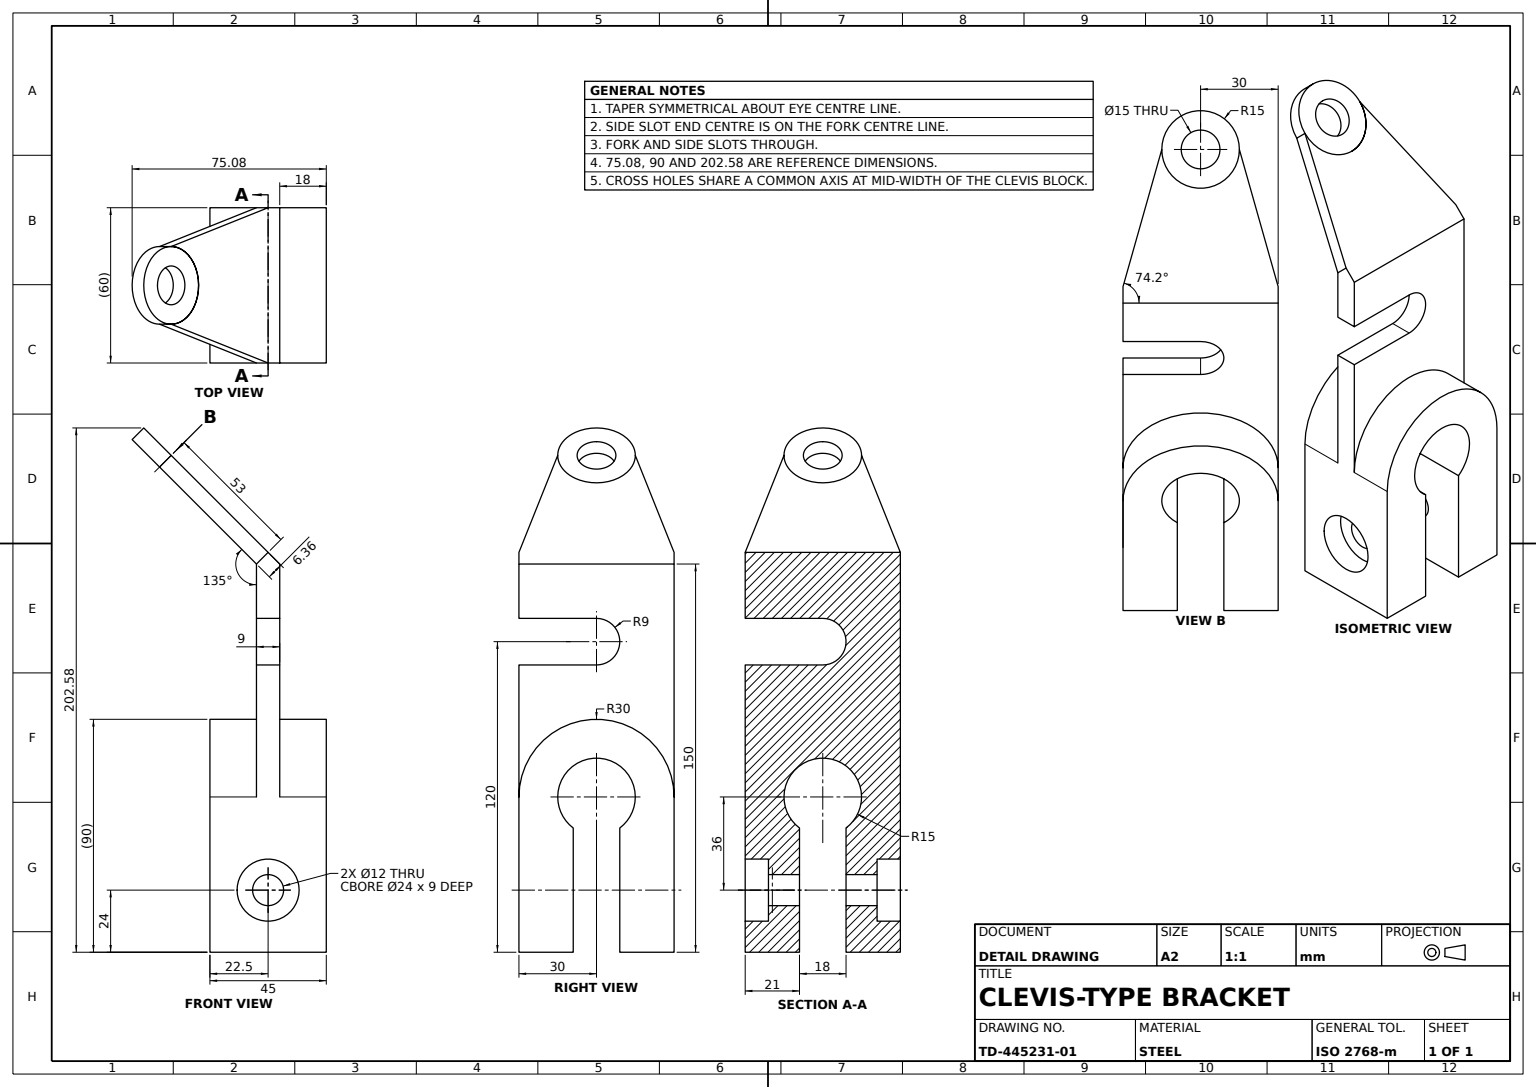
from build123d import *

# Parameters (mm, degrees)
CLEVIS_BLOCK_DEPTH         = 22.5
FORK_SLOT_DEPTH            = 64
SIDE_HOLE_A_PROFILE_R      = 12
SIDE_HOLE_A_DEPTH          = 9
SIDE_START                 = -9
SIDE_HOLE_B_PROFILE_R      = 12
SIDE_HOLE_B_DEPTH          = 9
CROSS_HOLE_PROFILE_R       = 6
CROSS_HOLE_DEPTH           = 51
ARM_PLATE_DEPTH            = 4.5
BRACKET_WEB_DEPTH          = 60
PIN_BOSS_PROFILE_R         = 15
PIN_BOSS_DEPTH             = 9
HOOK_SLOT_DEPTH            = 9
BOSS_START                 = -2
BOSS_RECESS_PROFILE_R      = 15
BOSS_RECESS_2MM_DEPTH      = 2
BOSS_START_2               = -16
BOSS_BORE_PROFILE_R        = 15
BOSS_BORE_DEPTH            = 16
BORE_INSERT_BOSS_PROFILE_R = 15
BORE_INSERT_BOSS_DEPTH     = 6.36
INSERT_BORE_PROFILE_R      = 7.5
INSERT_BORE_DEPTH          = 26.36
ARM_TRIM_CUT_DEPTH         = 26.36


with BuildPart() as part:
    # Clevis Block Profile → Clevis Block (new, symmetric)
    with BuildSketch(Plane.XY):
        with BuildLine():
            Line((0, 0), (30, 0))
            Line((30, 0), (30, 60))
            ThreePointArc((30, 60), (0, 90), (-30, 60))
            Line((-30, 60), (-30, 0))
            Line((-30, 0), (0, 0))
        make_face()
    extrude(amount=CLEVIS_BLOCK_DEPTH, both=True)

    # Fork Slot Profile → Fork Slot (cut)
    with BuildSketch(Plane.XY.offset(22.5)):
        with BuildLine():
            Line((0, 0), (9, 0))
            Line((9, 0), (9, 48))
            ThreePointArc((9, 48), (0, 75), (-9, 48))
            Line((-9, 48), (-9, 0))
            Line((-9, 0), (0, 0))
        make_face()
    extrude(amount=-FORK_SLOT_DEPTH, mode=Mode.SUBTRACT)

    # Side Hole A Profile → Side Hole A (cut)
    with BuildSketch(Plane.ZY.offset(30)):
        with Locations((0, 24)):
            Circle(SIDE_HOLE_A_PROFILE_R)
    extrude(amount=-SIDE_HOLE_A_DEPTH, mode=Mode.SUBTRACT)

    # Side Hole B Profile → Side Hole B (cut)
    with BuildSketch(Plane(origin=(30, 0, 0), x_dir=(0, 0, -1), z_dir=(1, 0, 0)).offset(SIDE_START)):
        with Locations(Location((0, 24, 0), (0, 0, 180))):
            Circle(SIDE_HOLE_B_PROFILE_R)
    extrude(amount=SIDE_HOLE_B_DEPTH, mode=Mode.SUBTRACT)

    # Cross Hole Profile → Cross Hole (cut)
    with BuildSketch(Plane(origin=(21, 0, 0), x_dir=(0, 0, -1), z_dir=(1, 0, 0))):
        with Locations(Location((0, 24, 0), (0, 0, 180))):
            Circle(CROSS_HOLE_PROFILE_R)
    extrude(amount=-CROSS_HOLE_DEPTH, mode=Mode.SUBTRACT)

    # Arm Plate Profile → Arm Plate (add, symmetric)
    with BuildSketch(Plane.XY):
        with BuildLine():
            Line((-30, 60), (-30, 150))
            Line((-30, 150), (30, 150))
            Line((30, 150), (30, 60))
            ThreePointArc((30, 60), (0, 90), (-30, 60))
        make_face()
    extrude(amount=ARM_PLATE_DEPTH, both=True)

    # Bracket Web Profile → Bracket Web (add)
    with BuildSketch(Plane(origin=(30, 0, 0), x_dir=(0, 0, -1), z_dir=(1, 0, 0))):
        Polygon((4.5, 150), (-32.976659403, 187.476659403), (-37.476659403, 191.976659403), (-41.976659403, 187.476659403), (-4.5, 150), align=None)
    extrude(amount=-BRACKET_WEB_DEPTH)

    # Pin Boss Profile → Pin Boss (add)
    with BuildSketch(Plane(origin=(0, 72.75, -72.75), x_dir=(1, 0, 0), z_dir=(0, -0.7071067811865479, 0.7071067811865472))):
        with Locations(Location((0, 162.247997693, 0), (0, 0, 270))):
            Circle(PIN_BOSS_PROFILE_R)
    extrude(amount=-PIN_BOSS_DEPTH)

    # Hook Slot Profile → Hook Slot (cut)
    with BuildSketch(Plane(origin=(0, 72.75, -72.75), x_dir=(1, 0, 0), z_dir=(0, -0.7071067811865479, 0.7071067811865472))):
        Polygon((-15, 162.247997693), (-30, 109.247997693), (-30, 162.247997693), align=None)
        Polygon((15, 162.247997693), (30, 109.247997693), (30, 162.247997693), align=None)
    extrude(amount=-HOOK_SLOT_DEPTH, mode=Mode.SUBTRACT)

    # Boss Recess Profile → Boss Recess 2mm (cut)
    with BuildSketch(Plane(origin=(0, 79.113961031, -79.113961031), x_dir=(1, 0, 0), z_dir=(0, 0.7071067811865478, -0.7071067811865472)).offset(BOSS_START)):
        with Locations(Location((0, -162.247997693, 0), (0, 0, 180))):
            Circle(BOSS_RECESS_PROFILE_R)
    extrude(amount=BOSS_RECESS_2MM_DEPTH, mode=Mode.SUBTRACT)

    # Boss Bore Profile → Boss Bore (cut)
    with BuildSketch(Plane(origin=(0, 77.699747468, -77.699747468), x_dir=(1, 0, 0), z_dir=(0, 0.7071067811865479, -0.7071067811865472)).offset(BOSS_START_2)):
        with Locations((0, -162.247997693)):
            Circle(BOSS_BORE_PROFILE_R)
    extrude(amount=BOSS_BORE_DEPTH, mode=Mode.SUBTRACT)

    # Bore Insert Boss Profile → Bore Insert Boss (add)
    with BuildSketch(Plane(origin=(0, 72.75, -72.75), x_dir=(1, 0, 0), z_dir=(0, -0.7071067811865479, 0.7071067811865472))):
        with Locations((0, 162.247997693)):
            Circle(BORE_INSERT_BOSS_PROFILE_R)
    extrude(amount=-BORE_INSERT_BOSS_DEPTH)

    # Insert Bore Profile → Insert Bore (cut)
    with BuildSketch(Plane(origin=(0, 72.75, -72.75), x_dir=(1, 0, 0), z_dir=(0, -0.7071067811865479, 0.7071067811865472))):
        with Locations(Location((0, 162.247997693, 0), (0, 0, 270))):
            Circle(INSERT_BORE_PROFILE_R)
    extrude(amount=-INSERT_BORE_DEPTH, mode=Mode.SUBTRACT)

    # Arm Trim Profile → Arm Trim Cut (cut)
    with BuildSketch(Plane.XY.offset(4.5)):
        with BuildLine():
            Line((0, 111), (30, 111))
            Line((30, 111), (30, 120))
            Line((30, 120), (30, 129))
            Line((30, 129), (0, 129))
            ThreePointArc((0, 129), (-9, 120), (0, 111))
        make_face()
    extrude(amount=-ARM_TRIM_CUT_DEPTH, mode=Mode.SUBTRACT)


solid = part.part
